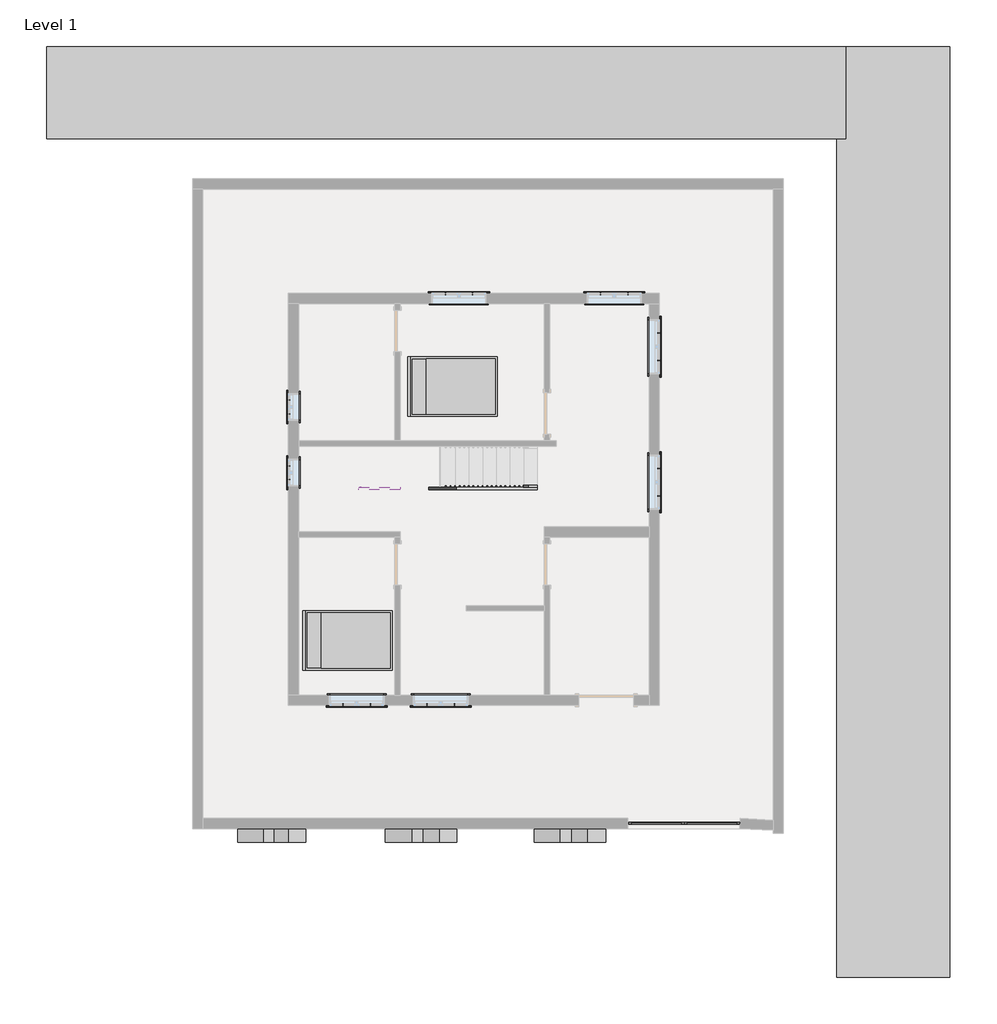
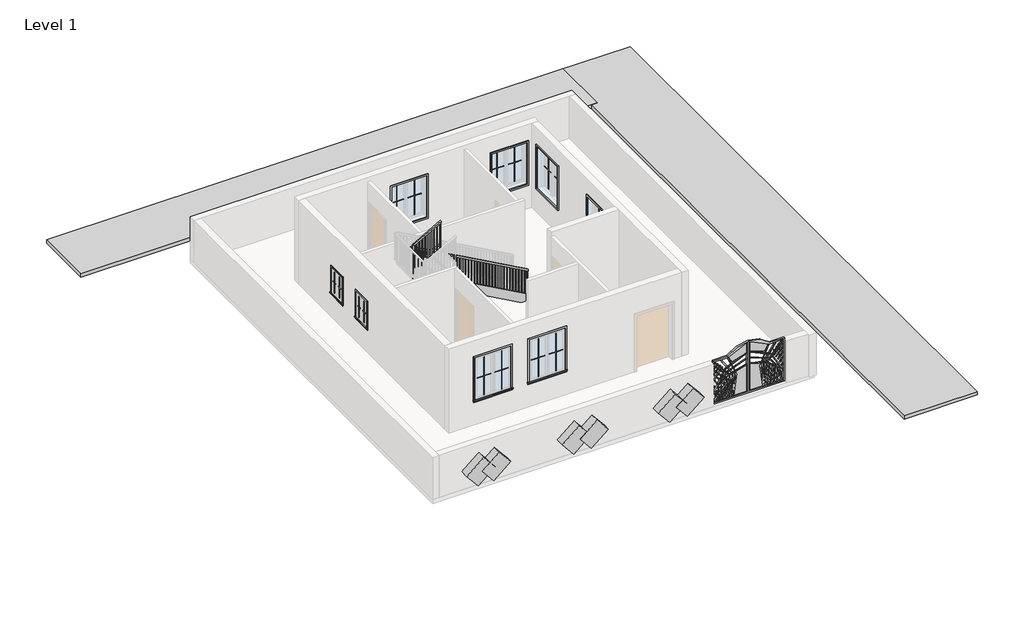
# One storey, part 2 of 2: 35 proxies, 3 members, 2 furniture elements, 1 railing.
"""IFC4 building model written with IfcOpenShell, lengths in millimetres."""

from ifc_helpers import new_model, si_unit, frame, origin, place, context, project, spatial, polyline, outline, extrude, faceted_brep, transform, mapped, element, save
from components import generic_models_6bc30956, generic_models_1_generic_models_1_8d9aa75c, generic_models_2_generic_models_2_aa56fe40, muntin_pattern_2x2_muntin_pattern_2x2_53152e2c, muntin_pattern_2x2_muntin_pattern_2x2_e8f3e573, muntin_pattern_2x2_muntin_pattern_2x2_6dad3731, muntin_pattern_2x2_muntin_pattern_2x2_a30a3345, trim_window_exterior_flat_with_sill_a665a915, trim_window_exterior_flat_with_sill_92b9b949, trim_window_interior_flat_picture_frame_d485c387, trim_window_interior_flat_picture_frame_3bb882cf, bed_17739_bed_17739_15c61121

model = new_model("IFC4")

# Units and contexts
model_context = context("Model", 3, world=origin())
ifc_project = project(units=[si_unit("LENGTHUNIT", "METRE", prefix="MILLI")], contexts=[model_context])

# Site, building, storey
site = spatial("IfcSite", under=ifc_project)
building = spatial("IfcBuilding", under=site)
storey = spatial("IfcBuildingStorey", under=building, Name="Level 1", Elevation=0.0)

# Proxies
placement = place(None, origin())
generic_models_shape = generic_models_6bc30956(model_context)
element("IfcBuildingElementProxy", 1, Name="Generic Models", at=placement, inside=storey, context=model_context, shape_type="MappedRepresentation", body=[
    mapped(generic_models_shape, transform((10047.0296029, 3046.038256, 0.0), x_axis=(1.0, 0.0, 0.0), y_axis=(0.0, 1.0, 0.0), z_axis=(0.0, 0.0, 1.0))),
])
generic_models_1_generic_models_1_shape = generic_models_1_generic_models_1_8d9aa75c(model_context)
element("IfcBuildingElementProxy", 2, Name="Generic Models 1 : Generic Models 1", ObjectType="Generic Models 1 : Generic Models 1", at=placement, inside=storey, context=model_context, shape_type="MappedRepresentation", body=[
    mapped(generic_models_1_generic_models_1_shape, transform((0.0, 0.0, 0.0), x_axis=(1.0, 0.0, 0.0), y_axis=(0.0, 1.0, 0.0), z_axis=(0.0, 0.0, 1.0))),
])
generic_models_2_generic_models_2_shape = generic_models_2_generic_models_2_aa56fe40(model_context)
element("IfcBuildingElementProxy", 3, Name="Generic Models 2 : Generic Models 2", ObjectType="Generic Models 2 : Generic Models 2", at=placement, inside=storey, context=model_context, shape_type="MappedRepresentation", body=[
    mapped(generic_models_2_generic_models_2_shape, transform((0.0, 0.0, 0.0), x_axis=(1.0, 0.0, 0.0), y_axis=(0.0, 1.0, 0.0), z_axis=(0.0, 0.0, 1.0))),
])
muntin_pattern_2x2_muntin_pattern_2x2_shape = muntin_pattern_2x2_muntin_pattern_2x2_53152e2c(model_context)
element("IfcBuildingElementProxy", 4, Name="Muntin Pattern_2x2 : Muntin Pattern_2x2", ObjectType="Muntin Pattern_2x2 : Muntin Pattern_2x2", at=placement, inside=storey, context=model_context, shape_type="MappedRepresentation", body=[
    mapped(muntin_pattern_2x2_muntin_pattern_2x2_shape, transform((1279.525, 12101.9997886, 984.25), x_axis=(0.0, 1.0, 0.0), y_axis=(-1.0, 0.0, 0.0), z_axis=(0.0, 0.0, 1.0))),
])
element("IfcBuildingElementProxy", 5, Name="Muntin Pattern_2x2 : Muntin Pattern_2x2", ObjectType="Muntin Pattern_2x2 : Muntin Pattern_2x2", at=placement, inside=storey, context=model_context, shape_type="MappedRepresentation", body=[
    mapped(muntin_pattern_2x2_muntin_pattern_2x2_shape, transform((1279.525, 10644.6747886, 984.25), x_axis=(0.0, 1.0, 0.0), y_axis=(-1.0, 0.0, 0.0), z_axis=(0.0, 0.0, 1.0))),
])
muntin_pattern_2x2_muntin_pattern_2x2_2_shape = muntin_pattern_2x2_muntin_pattern_2x2_e8f3e573(model_context)
element("IfcBuildingElementProxy", 6, Name="Muntin Pattern_2x2 : Muntin Pattern_2x2", ObjectType="Muntin Pattern_2x2 : Muntin Pattern_2x2", at=placement, inside=storey, context=model_context, shape_type="MappedRepresentation", body=[
    mapped(muntin_pattern_2x2_muntin_pattern_2x2_2_shape, transform((1279.525, 12403.6247886, 984.25), x_axis=(0.0, -1.0, 0.0), y_axis=(1.0, 0.0, 0.0), z_axis=(0.0, 0.0, 1.0))),
])
element("IfcBuildingElementProxy", 7, Name="Muntin Pattern_2x2 : Muntin Pattern_2x2", ObjectType="Muntin Pattern_2x2 : Muntin Pattern_2x2", at=placement, inside=storey, context=model_context, shape_type="MappedRepresentation", body=[
    mapped(muntin_pattern_2x2_muntin_pattern_2x2_2_shape, transform((1279.525, 10946.2997886, 984.25), x_axis=(0.0, -1.0, 0.0), y_axis=(1.0, 0.0, 0.0), z_axis=(0.0, 0.0, 1.0))),
])
muntin_pattern_2x2_muntin_pattern_2x2_3_shape = muntin_pattern_2x2_muntin_pattern_2x2_6dad3731(model_context)
element("IfcBuildingElementProxy", 8, Name="Muntin Pattern_2x2 : Muntin Pattern_2x2", ObjectType="Muntin Pattern_2x2 : Muntin Pattern_2x2", at=placement, inside=storey, context=model_context, shape_type="MappedRepresentation", body=[
    mapped(muntin_pattern_2x2_muntin_pattern_2x2_3_shape, transform((9490.075, 13892.6997886, 984.25), x_axis=(0.0, -1.0, 0.0), y_axis=(1.0, 0.0, 0.0), z_axis=(0.0, 0.0, 1.0))),
])
element("IfcBuildingElementProxy", 9, Name="Muntin Pattern_2x2 : Muntin Pattern_2x2", ObjectType="Muntin Pattern_2x2 : Muntin Pattern_2x2", at=placement, inside=storey, context=model_context, shape_type="MappedRepresentation", body=[
    mapped(muntin_pattern_2x2_muntin_pattern_2x2_3_shape, transform((8193.0875, 14767.4122886, 984.25), x_axis=(1.0, 0.0, 0.0), y_axis=(0.0, 1.0, 0.0), z_axis=(0.0, 0.0, 1.0))),
])
element("IfcBuildingElementProxy", 10, Name="Muntin Pattern_2x2 : Muntin Pattern_2x2", ObjectType="Muntin Pattern_2x2 : Muntin Pattern_2x2", at=placement, inside=storey, context=model_context, shape_type="MappedRepresentation", body=[
    mapped(muntin_pattern_2x2_muntin_pattern_2x2_3_shape, transform((4749.8, 14767.4122886, 984.25), x_axis=(1.0, 0.0, 0.0), y_axis=(0.0, 1.0, 0.0), z_axis=(0.0, 0.0, 1.0))),
])
element("IfcBuildingElementProxy", 11, Name="Muntin Pattern_2x2 : Muntin Pattern_2x2", ObjectType="Muntin Pattern_2x2 : Muntin Pattern_2x2", at=placement, inside=storey, context=model_context, shape_type="MappedRepresentation", body=[
    mapped(muntin_pattern_2x2_muntin_pattern_2x2_3_shape, transform((9490.075, 10889.1497886, 984.25), x_axis=(0.0, -1.0, 0.0), y_axis=(1.0, 0.0, 0.0), z_axis=(0.0, 0.0, 1.0))),
])
element("IfcBuildingElementProxy", 12, Name="Muntin Pattern_2x2 : Muntin Pattern_2x2", ObjectType="Muntin Pattern_2x2 : Muntin Pattern_2x2", at=placement, inside=storey, context=model_context, shape_type="MappedRepresentation", body=[
    mapped(muntin_pattern_2x2_muntin_pattern_2x2_3_shape, transform((4950.6207347, 5642.4622886, 984.25), x_axis=(-1.0, 0.0, 0.0), y_axis=(0.0, -1.0, 0.0), z_axis=(0.0, 0.0, 1.0))),
])
element("IfcBuildingElementProxy", 13, Name="Muntin Pattern_2x2 : Muntin Pattern_2x2", ObjectType="Muntin Pattern_2x2 : Muntin Pattern_2x2", at=placement, inside=storey, context=model_context, shape_type="MappedRepresentation", body=[
    mapped(muntin_pattern_2x2_muntin_pattern_2x2_3_shape, transform((3086.1019847, 5642.4622886, 984.25), x_axis=(-1.0, 0.0, 0.0), y_axis=(0.0, -1.0, 0.0), z_axis=(0.0, 0.0, 1.0))),
])
muntin_pattern_2x2_muntin_pattern_2x2_4_shape = muntin_pattern_2x2_muntin_pattern_2x2_a30a3345(model_context)
element("IfcBuildingElementProxy", 14, Name="Muntin Pattern_2x2 : Muntin Pattern_2x2", ObjectType="Muntin Pattern_2x2 : Muntin Pattern_2x2", at=placement, inside=storey, context=model_context, shape_type="MappedRepresentation", body=[
    mapped(muntin_pattern_2x2_muntin_pattern_2x2_4_shape, transform((9490.075, 13286.2747886, 984.25), x_axis=(0.0, 1.0, 0.0), y_axis=(-1.0, 0.0, 0.0), z_axis=(0.0, 0.0, 1.0))),
])
element("IfcBuildingElementProxy", 15, Name="Muntin Pattern_2x2 : Muntin Pattern_2x2", ObjectType="Muntin Pattern_2x2 : Muntin Pattern_2x2", at=placement, inside=storey, context=model_context, shape_type="MappedRepresentation", body=[
    mapped(muntin_pattern_2x2_muntin_pattern_2x2_4_shape, transform((8799.5125, 14767.4122886, 984.25), x_axis=(-1.0, 0.0, 0.0), y_axis=(0.0, -1.0, 0.0), z_axis=(0.0, 0.0, 1.0))),
])
element("IfcBuildingElementProxy", 16, Name="Muntin Pattern_2x2 : Muntin Pattern_2x2", ObjectType="Muntin Pattern_2x2 : Muntin Pattern_2x2", at=placement, inside=storey, context=model_context, shape_type="MappedRepresentation", body=[
    mapped(muntin_pattern_2x2_muntin_pattern_2x2_4_shape, transform((5356.225, 14767.4122886, 984.25), x_axis=(-1.0, 0.0, 0.0), y_axis=(0.0, -1.0, 0.0), z_axis=(0.0, 0.0, 1.0))),
])
element("IfcBuildingElementProxy", 17, Name="Muntin Pattern_2x2 : Muntin Pattern_2x2", ObjectType="Muntin Pattern_2x2 : Muntin Pattern_2x2", at=placement, inside=storey, context=model_context, shape_type="MappedRepresentation", body=[
    mapped(muntin_pattern_2x2_muntin_pattern_2x2_4_shape, transform((9490.075, 10282.7247886, 984.25), x_axis=(0.0, 1.0, 0.0), y_axis=(-1.0, 0.0, 0.0), z_axis=(0.0, 0.0, 1.0))),
])
element("IfcBuildingElementProxy", 18, Name="Muntin Pattern_2x2 : Muntin Pattern_2x2", ObjectType="Muntin Pattern_2x2 : Muntin Pattern_2x2", at=placement, inside=storey, context=model_context, shape_type="MappedRepresentation", body=[
    mapped(muntin_pattern_2x2_muntin_pattern_2x2_4_shape, transform((4344.1957347, 5642.4622886, 984.25), x_axis=(1.0, 0.0, 0.0), y_axis=(0.0, 1.0, 0.0), z_axis=(0.0, 0.0, 1.0))),
])
element("IfcBuildingElementProxy", 19, Name="Muntin Pattern_2x2 : Muntin Pattern_2x2", ObjectType="Muntin Pattern_2x2 : Muntin Pattern_2x2", at=placement, inside=storey, context=model_context, shape_type="MappedRepresentation", body=[
    mapped(muntin_pattern_2x2_muntin_pattern_2x2_4_shape, transform((2479.6769847, 5642.4622886, 984.25), x_axis=(1.0, 0.0, 0.0), y_axis=(0.0, 1.0, 0.0), z_axis=(0.0, 0.0, 1.0))),
])
trim_window_exterior_flat_with_sill_shape = trim_window_exterior_flat_with_sill_a665a915(model_context)
element("IfcBuildingElementProxy", 20, Name="Trim-Window-Exterior-Flat : with Sill", ObjectType="Trim-Window-Exterior-Flat : with Sill", at=placement, inside=storey, context=model_context, shape_type="MappedRepresentation", body=[
    mapped(trim_window_exterior_flat_with_sill_shape, transform((1270.0, 12252.8122886, 1828.8), x_axis=(0.0, -1.0, 0.0), y_axis=(0.0, 0.0, 1.0), z_axis=(-1.0, 0.0, 0.0))),
])
element("IfcBuildingElementProxy", 21, Name="Trim-Window-Exterior-Flat : with Sill", ObjectType="Trim-Window-Exterior-Flat : with Sill", at=placement, inside=storey, context=model_context, shape_type="MappedRepresentation", body=[
    mapped(trim_window_exterior_flat_with_sill_shape, transform((1270.0, 10795.4872886, 1828.8), x_axis=(0.0, -1.0, 0.0), y_axis=(0.0, 0.0, 1.0), z_axis=(-1.0, 0.0, 0.0))),
])
trim_window_exterior_flat_with_sill_2_shape = trim_window_exterior_flat_with_sill_92b9b949(model_context)
element("IfcBuildingElementProxy", 22, Name="Trim-Window-Exterior-Flat : with Sill", ObjectType="Trim-Window-Exterior-Flat : with Sill", at=placement, inside=storey, context=model_context, shape_type="MappedRepresentation", body=[
    mapped(trim_window_exterior_flat_with_sill_2_shape, transform((9499.6, 13589.4872886, 2438.4), x_axis=(0.0, 1.0, 0.0), y_axis=(0.0, 0.0, 1.0), z_axis=(1.0, 0.0, 0.0))),
])
element("IfcBuildingElementProxy", 23, Name="Trim-Window-Exterior-Flat : with Sill", ObjectType="Trim-Window-Exterior-Flat : with Sill", at=placement, inside=storey, context=model_context, shape_type="MappedRepresentation", body=[
    mapped(trim_window_exterior_flat_with_sill_2_shape, transform((8496.3, 14776.9372886, 2438.4), x_axis=(-1.0, 0.0, 0.0), y_axis=(0.0, 0.0, 1.0), z_axis=(0.0, 1.0, 0.0))),
])
element("IfcBuildingElementProxy", 24, Name="Trim-Window-Exterior-Flat : with Sill", ObjectType="Trim-Window-Exterior-Flat : with Sill", at=placement, inside=storey, context=model_context, shape_type="MappedRepresentation", body=[
    mapped(trim_window_exterior_flat_with_sill_2_shape, transform((5053.0125, 14776.9372886, 2438.4), x_axis=(-1.0, 0.0, 0.0), y_axis=(0.0, 0.0, 1.0), z_axis=(0.0, 1.0, 0.0))),
])
element("IfcBuildingElementProxy", 25, Name="Trim-Window-Exterior-Flat : with Sill", ObjectType="Trim-Window-Exterior-Flat : with Sill", at=placement, inside=storey, context=model_context, shape_type="MappedRepresentation", body=[
    mapped(trim_window_exterior_flat_with_sill_2_shape, transform((9499.6, 10585.9372886, 2438.4), x_axis=(0.0, 1.0, 0.0), y_axis=(0.0, 0.0, 1.0), z_axis=(1.0, 0.0, 0.0))),
])
element("IfcBuildingElementProxy", 26, Name="Trim-Window-Exterior-Flat : with Sill", ObjectType="Trim-Window-Exterior-Flat : with Sill", at=placement, inside=storey, context=model_context, shape_type="MappedRepresentation", body=[
    mapped(trim_window_exterior_flat_with_sill_2_shape, transform((4647.4082347, 5632.9372886, 2438.4), x_axis=(1.0, 0.0, 0.0), y_axis=(0.0, 0.0, 1.0), z_axis=(0.0, -1.0, 0.0))),
])
element("IfcBuildingElementProxy", 27, Name="Trim-Window-Exterior-Flat : with Sill", ObjectType="Trim-Window-Exterior-Flat : with Sill", at=placement, inside=storey, context=model_context, shape_type="MappedRepresentation", body=[
    mapped(trim_window_exterior_flat_with_sill_2_shape, transform((2782.8894847, 5632.9372886, 2438.4), x_axis=(1.0, 0.0, 0.0), y_axis=(0.0, 0.0, 1.0), z_axis=(0.0, -1.0, 0.0))),
])
trim_window_interior_flat_picture_frame_shape = trim_window_interior_flat_picture_frame_d485c387(model_context)
element("IfcBuildingElementProxy", 28, Name="Trim-Window-Interior-Flat : Picture Frame", ObjectType="Trim-Window-Interior-Flat : Picture Frame", at=placement, inside=storey, context=model_context, shape_type="MappedRepresentation", body=[
    mapped(trim_window_interior_flat_picture_frame_shape, transform((1498.6, 12252.8122886, 1828.8), x_axis=(0.0, 1.0, 0.0), y_axis=(0.0, 0.0, 1.0), z_axis=(1.0, 0.0, 0.0))),
])
element("IfcBuildingElementProxy", 29, Name="Trim-Window-Interior-Flat : Picture Frame", ObjectType="Trim-Window-Interior-Flat : Picture Frame", at=placement, inside=storey, context=model_context, shape_type="MappedRepresentation", body=[
    mapped(trim_window_interior_flat_picture_frame_shape, transform((1498.6, 10795.4872886, 1828.8), x_axis=(0.0, 1.0, 0.0), y_axis=(0.0, 0.0, 1.0), z_axis=(1.0, 0.0, 0.0))),
])
trim_window_interior_flat_picture_frame_2_shape = trim_window_interior_flat_picture_frame_3bb882cf(model_context)
element("IfcBuildingElementProxy", 30, Name="Trim-Window-Interior-Flat : Picture Frame", ObjectType="Trim-Window-Interior-Flat : Picture Frame", at=placement, inside=storey, context=model_context, shape_type="MappedRepresentation", body=[
    mapped(trim_window_interior_flat_picture_frame_2_shape, transform((9271.0, 13589.4872886, 2438.4), x_axis=(0.0, -1.0, 0.0), y_axis=(0.0, 0.0, 1.0), z_axis=(-1.0, 0.0, 0.0))),
])
element("IfcBuildingElementProxy", 31, Name="Trim-Window-Interior-Flat : Picture Frame", ObjectType="Trim-Window-Interior-Flat : Picture Frame", at=placement, inside=storey, context=model_context, shape_type="MappedRepresentation", body=[
    mapped(trim_window_interior_flat_picture_frame_2_shape, transform((8496.3, 14548.3372886, 2438.4), x_axis=(1.0, 0.0, 0.0), y_axis=(0.0, 0.0, 1.0), z_axis=(0.0, -1.0, 0.0))),
])
element("IfcBuildingElementProxy", 32, Name="Trim-Window-Interior-Flat : Picture Frame", ObjectType="Trim-Window-Interior-Flat : Picture Frame", at=placement, inside=storey, context=model_context, shape_type="MappedRepresentation", body=[
    mapped(trim_window_interior_flat_picture_frame_2_shape, transform((5053.0125, 14548.3372886, 2438.4), x_axis=(1.0, 0.0, 0.0), y_axis=(0.0, 0.0, 1.0), z_axis=(0.0, -1.0, 0.0))),
])
element("IfcBuildingElementProxy", 33, Name="Trim-Window-Interior-Flat : Picture Frame", ObjectType="Trim-Window-Interior-Flat : Picture Frame", at=placement, inside=storey, context=model_context, shape_type="MappedRepresentation", body=[
    mapped(trim_window_interior_flat_picture_frame_2_shape, transform((9271.0, 10585.9372886, 2438.4), x_axis=(0.0, -1.0, 0.0), y_axis=(0.0, 0.0, 1.0), z_axis=(-1.0, 0.0, 0.0))),
])
element("IfcBuildingElementProxy", 34, Name="Trim-Window-Interior-Flat : Picture Frame", ObjectType="Trim-Window-Interior-Flat : Picture Frame", at=placement, inside=storey, context=model_context, shape_type="MappedRepresentation", body=[
    mapped(trim_window_interior_flat_picture_frame_2_shape, transform((4647.4082347, 5861.5372886, 2438.4), x_axis=(-1.0, 0.0, 0.0), y_axis=(0.0, 0.0, 1.0), z_axis=(0.0, 1.0, 0.0))),
])
element("IfcBuildingElementProxy", 35, Name="Trim-Window-Interior-Flat : Picture Frame", ObjectType="Trim-Window-Interior-Flat : Picture Frame", at=placement, inside=storey, context=model_context, shape_type="MappedRepresentation", body=[
    mapped(trim_window_interior_flat_picture_frame_2_shape, transform((2782.8894847, 5861.5372886, 2438.4), x_axis=(-1.0, 0.0, 0.0), y_axis=(0.0, 0.0, 1.0), z_axis=(0.0, 1.0, 0.0))),
])

# Furniture
bed_17739_bed_17739_shape = bed_17739_bed_17739_15c61121(model_context)
element("IfcFurniture", 36, ObjectType="Bed_17739 : Bed_17739", at=placement, inside=storey, context=model_context, shape_type="MappedRepresentation", body=[
    mapped(bed_17739_bed_17739_shape, transform((4933.95, 12706.8372886, 0.0), x_axis=(0.0, 1.0, 0.0), y_axis=(-1.0, 0.0, 0.0), z_axis=(0.0, 0.0, 1.0))),
])
element("IfcFurniture", 37, ObjectType="Bed_17739 : Bed_17739", at=placement, inside=storey, context=model_context, shape_type="MappedRepresentation", body=[
    mapped(bed_17739_bed_17739_shape, transform((2603.5, 7074.3872886, 0.0), x_axis=(0.0, 1.0, 0.0), y_axis=(-1.0, 0.0, 0.0), z_axis=(0.0, 0.0, 1.0))),
])

# Members
element("IfcMember", 38, ObjectType="Stringer - 2\" Width", at=placement, inside=storey, context=model_context, shape_type="SweptSolid", body=[
    extrude(outline(polyline([(0.0, 6794.5), (207.5983948, 6794.5), (2380.7095059, 2882.9), (2032.0308318, 2882.9), (0.0, 6540.5554972), (0.0, 6794.5)])), frame((0.0, 10420.8372886, 0.0), z_axis=(0.0, 1.0, 0.0), x_axis=(0.0, 0.0, 1.0)), (0.0, 0.0, 1.0), 50.8),
])
element("IfcMember", 39, ObjectType="Stringer - 2\" Width", at=placement, inside=storey, context=model_context, shape_type="SweptSolid", body=[
    extrude(outline(polyline([(2832.1, 10471.6372886), (2882.9, 10471.6372886), (2882.9, 10469.0972886), (2832.1, 10469.0972886), (2832.1, 10471.6372886)])), frame((0.0, 0.0, 2142.0666667), z_axis=(0.0, 0.0, 1.0), x_axis=(1.0, 0.0, 0.0)), (0.0, 0.0, 1.0), 304.8),
])
element("IfcMember", 40, ObjectType="Stringer - 2\" Width", at=placement, inside=storey, context=model_context, shape_type="SweptSolid", body=[
    extrude(outline(polyline([(2578.2650614, 2832.1), (2229.5863873, 2832.1), (2737.5874899, 3746.5019847), (3086.266164, 3746.5019847), (2578.2650614, 2832.1)])), frame((0.0, 10418.2972886, 0.0), z_axis=(0.0, 1.0, 0.0), x_axis=(0.0, 0.0, 1.0)), (0.0, 0.0, 1.0), 50.8),
])

# Railing
element("IfcRailing", 41, ObjectType="Handrail - Rectangular", at=placement, inside=storey, context=model_context, shape_type="SolidModel", body=[
    faceted_brep([(6794.5, 10471.6372886, 1083.7333333), (6794.5, 10471.6372886, 1025.620221), (6794.5, 10522.4372886, 1025.620221), (6794.5, 10522.4372886, 1083.7333333), (2908.3, 10471.6372886, 3242.7333333), (2857.5, 10471.6372886, 3212.8424432), (2857.5, 10522.4372886, 3212.8424432), (2908.3, 10522.4372886, 3242.7333333), (2908.3, 10471.6372886, 3285.0666667), (2857.5, 10471.6372886, 3234.2666667), (2857.5, 10522.4372886, 3234.2666667), (2908.3, 10522.4372886, 3285.0666667), (2832.1, 10471.6372886, 3285.0666667), (2832.1, 10471.6372886, 3234.2666667), (2781.3, 10522.4372886, 3234.2666667), (2781.3, 10522.4372886, 3285.0666667), (2832.1, 10395.4372886, 3285.0666667), (2832.1, 10395.4372886, 3234.2666667), (2781.3, 10395.4372886, 3234.2666667), (2781.3, 10395.4372886, 3285.0666667), (2832.1, 10392.8972886, 3285.0666667), (2781.3, 10392.8972886, 3285.0666667), (2781.3, 10392.8972886, 3234.2666667), (2832.1, 10392.8972886, 3234.2666667)], [[[0, 1, 2, 3]], [[1, 0, 4, 5]], [[2, 1, 5, 6]], [[3, 2, 6, 7]], [[0, 3, 7, 4]], [[5, 4, 8, 9]], [[6, 5, 9, 10]], [[7, 6, 10, 11]], [[4, 7, 11, 8]], [[9, 8, 12, 13]], [[10, 9, 13, 14]], [[11, 10, 14, 15]], [[8, 11, 15, 12]], [[13, 12, 16, 17]], [[14, 13, 17, 18]], [[15, 14, 18, 19]], [[12, 15, 19, 16]], [[20, 21, 22, 23]], [[17, 16, 20, 23]], [[18, 17, 23, 22]], [[19, 18, 22, 21]], [[16, 19, 21, 20]]]),
    faceted_brep([(2832.1, 10418.2972886, 3285.0666667), (2832.1, 10367.4972886, 3234.2666667), (2781.3, 10367.4972886, 3234.2666667), (2781.3, 10418.2972886, 3285.0666667), (2832.1, 10418.2972886, 3396.2869174), (2781.3, 10418.2972886, 3426.177839), (2781.3, 10367.4972886, 3426.177839), (2832.1, 10367.4972886, 3396.2869174)], [[[0, 1, 2, 3]], [[4, 5, 6, 7]], [[1, 0, 4, 7]], [[2, 1, 7, 6]], [[3, 2, 6, 5]], [[0, 3, 5, 4]]]),
    faceted_brep([(2781.3, 10418.2972886, 3426.177839), (2832.1, 10418.2972886, 3396.2869174), (2832.1, 10367.4972886, 3396.2869174), (2781.3, 10367.4972886, 3426.177839), (3746.5019847, 10418.2972886, 3962.4), (3746.5019847, 10367.4972886, 3962.4), (3746.5019847, 10367.4972886, 3904.2869174), (3746.5019847, 10418.2972886, 3904.2869174)], [[[0, 1, 2, 3]], [[4, 5, 6, 7]], [[1, 0, 4, 7]], [[2, 1, 7, 6]], [[3, 2, 6, 5]], [[0, 3, 5, 4]]]),
    extrude(outline(polyline([(3884.8838142, 3711.575), (2878.6666667, 3711.575), (2878.6666667, 3730.625), (3895.4671246, 3730.625), (3884.8838142, 3711.575)])), frame((0.0, 10383.3722886, 0.0), z_axis=(0.0, 1.0, 0.0), x_axis=(0.0, 0.0, 1.0)), (0.0, 0.0, 1.0), 19.05),
    extrude(outline(polyline([(3828.4394923, 3609.975), (2878.6666667, 3609.975), (2878.6666667, 3629.025), (3839.0228026, 3629.025), (3828.4394923, 3609.975)])), frame((0.0, 10383.3722886, 0.0), z_axis=(0.0, 1.0, 0.0), x_axis=(0.0, 0.0, 1.0)), (0.0, 0.0, 1.0), 19.05),
    extrude(outline(polyline([(3771.9951703, 3508.375), (2878.6666667, 3508.375), (2878.6666667, 3527.425), (3782.5784807, 3527.425), (3771.9951703, 3508.375)])), frame((0.0, 10383.3722886, 0.0), z_axis=(0.0, 1.0, 0.0), x_axis=(0.0, 0.0, 1.0)), (0.0, 0.0, 1.0), 19.05),
    extrude(outline(polyline([(3715.5504809, 3406.775), (2709.3333333, 3406.775), (2709.3333333, 3425.825), (3726.1337912, 3425.825), (3715.5504809, 3406.775)])), frame((0.0, 10383.3722886, 0.0), z_axis=(0.0, 1.0, 0.0), x_axis=(0.0, 0.0, 1.0)), (0.0, 0.0, 1.0), 19.05),
    extrude(outline(polyline([(3659.1061589, 3305.175), (2709.3333333, 3305.175), (2709.3333333, 3324.225), (3669.6894693, 3324.225), (3659.1061589, 3305.175)])), frame((0.0, 10383.3722886, 0.0), z_axis=(0.0, 1.0, 0.0), x_axis=(0.0, 0.0, 1.0)), (0.0, 0.0, 1.0), 19.05),
    extrude(outline(polyline([(3602.661837, 3203.575), (2709.3333333, 3203.575), (2709.3333333, 3222.625), (3613.2451474, 3222.625), (3602.661837, 3203.575)])), frame((0.0, 10383.3722886, 0.0), z_axis=(0.0, 1.0, 0.0), x_axis=(0.0, 0.0, 1.0)), (0.0, 0.0, 1.0), 19.05),
    extrude(outline(polyline([(3546.2171475, 3101.975), (2540.0, 3101.975), (2540.0, 3121.025), (3556.8004579, 3121.025), (3546.2171475, 3101.975)])), frame((0.0, 10383.3722886, 0.0), z_axis=(0.0, 1.0, 0.0), x_axis=(0.0, 0.0, 1.0)), (0.0, 0.0, 1.0), 19.05),
    extrude(outline(polyline([(3489.7728256, 3000.375), (2540.0, 3000.375), (2540.0, 3019.425), (3500.356136, 3019.425), (3489.7728256, 3000.375)])), frame((0.0, 10383.3722886, 0.0), z_axis=(0.0, 1.0, 0.0), x_axis=(0.0, 0.0, 1.0)), (0.0, 0.0, 1.0), 19.05),
    extrude(outline(polyline([(3433.3285037, 2898.775), (2540.0, 2898.775), (2540.0, 2917.825), (3443.911814, 2917.825), (3433.3285037, 2898.775)])), frame((0.0, 10383.3722886, 0.0), z_axis=(0.0, 1.0, 0.0), x_axis=(0.0, 0.0, 1.0)), (0.0, 0.0, 1.0), 19.05),
    extrude(outline(polyline([(2816.225, 10404.9622886), (2816.225, 10385.9122886), (2797.175, 10385.9122886), (2797.175, 10404.9622886), (2816.225, 10404.9622886)])), frame((0.0, 0.0, 2370.6666667), z_axis=(0.0, 0.0, 1.0), x_axis=(1.0, 0.0, 0.0)), (0.0, 0.0, 1.0), 863.6),
    extrude(outline(polyline([(2841.625, 10487.5122886), (2822.575, 10487.5122886), (2822.575, 10506.5622886), (2841.625, 10506.5622886), (2841.625, 10487.5122886)])), frame((0.0, 0.0, 2370.6666667), z_axis=(0.0, 0.0, 1.0), x_axis=(1.0, 0.0, 0.0)), (0.0, 0.0, 1.0), 863.6),
    extrude(outline(polyline([(3175.8007765, 2924.175), (2201.3333333, 2924.175), (2201.3333333, 2943.225), (3165.2174432, 2943.225), (3175.8007765, 2924.175)])), frame((0.0, 10487.5122886, 0.0), z_axis=(0.0, 1.0, 0.0), x_axis=(0.0, 0.0, 1.0)), (0.0, 0.0, 1.0), 19.05),
    extrude(outline(polyline([(3119.3563321, 3025.775), (2201.3333333, 3025.775), (2201.3333333, 3044.825), (3108.7729988, 3044.825), (3119.3563321, 3025.775)])), frame((0.0, 10487.5122886, 0.0), z_axis=(0.0, 1.0, 0.0), x_axis=(0.0, 0.0, 1.0)), (0.0, 0.0, 1.0), 19.05),
    extrude(outline(polyline([(3062.9118876, 3127.375), (2201.3333333, 3127.375), (2201.3333333, 3146.425), (3052.3285543, 3146.425), (3062.9118876, 3127.375)])), frame((0.0, 10487.5122886, 0.0), z_axis=(0.0, 1.0, 0.0), x_axis=(0.0, 0.0, 1.0)), (0.0, 0.0, 1.0), 19.05),
    extrude(outline(polyline([(3006.4674432, 3228.975), (2032.0, 3228.975), (2032.0, 3248.025), (2995.8841099, 3248.025), (3006.4674432, 3228.975)])), frame((0.0, 10487.5122886, 0.0), z_axis=(0.0, 1.0, 0.0), x_axis=(0.0, 0.0, 1.0)), (0.0, 0.0, 1.0), 19.05),
    extrude(outline(polyline([(2950.0229988, 3330.575), (2032.0, 3330.575), (2032.0, 3349.625), (2939.4396654, 3349.625), (2950.0229988, 3330.575)])), frame((0.0, 10487.5122886, 0.0), z_axis=(0.0, 1.0, 0.0), x_axis=(0.0, 0.0, 1.0)), (0.0, 0.0, 1.0), 19.05),
    extrude(outline(polyline([(2893.5785543, 3432.175), (2032.0, 3432.175), (2032.0, 3451.225), (2882.995221, 3451.225), (2893.5785543, 3432.175)])), frame((0.0, 10487.5122886, 0.0), z_axis=(0.0, 1.0, 0.0), x_axis=(0.0, 0.0, 1.0)), (0.0, 0.0, 1.0), 19.05),
    extrude(outline(polyline([(2837.1341099, 3533.775), (1862.6666667, 3533.775), (1862.6666667, 3552.825), (2826.5507765, 3552.825), (2837.1341099, 3533.775)])), frame((0.0, 10487.5122886, 0.0), z_axis=(0.0, 1.0, 0.0), x_axis=(0.0, 0.0, 1.0)), (0.0, 0.0, 1.0), 19.05),
    extrude(outline(polyline([(2780.6896654, 3635.375), (1862.6666667, 3635.375), (1862.6666667, 3654.425), (2770.1063321, 3654.425), (2780.6896654, 3635.375)])), frame((0.0, 10487.5122886, 0.0), z_axis=(0.0, 1.0, 0.0), x_axis=(0.0, 0.0, 1.0)), (0.0, 0.0, 1.0), 19.05),
    extrude(outline(polyline([(2724.245221, 3736.975), (1862.6666667, 3736.975), (1862.6666667, 3756.025), (2713.6618876, 3756.025), (2724.245221, 3736.975)])), frame((0.0, 10487.5122886, 0.0), z_axis=(0.0, 1.0, 0.0), x_axis=(0.0, 0.0, 1.0)), (0.0, 0.0, 1.0), 19.05),
    extrude(outline(polyline([(2667.8007765, 3838.575), (1693.3333333, 3838.575), (1693.3333333, 3857.625), (2657.2174432, 3857.625), (2667.8007765, 3838.575)])), frame((0.0, 10487.5122886, 0.0), z_axis=(0.0, 1.0, 0.0), x_axis=(0.0, 0.0, 1.0)), (0.0, 0.0, 1.0), 19.05),
    extrude(outline(polyline([(2611.3563321, 3940.175), (1693.3333333, 3940.175), (1693.3333333, 3959.225), (2600.7729988, 3959.225), (2611.3563321, 3940.175)])), frame((0.0, 10487.5122886, 0.0), z_axis=(0.0, 1.0, 0.0), x_axis=(0.0, 0.0, 1.0)), (0.0, 0.0, 1.0), 19.05),
    extrude(outline(polyline([(2554.9118876, 4041.775), (1693.3333333, 4041.775), (1693.3333333, 4060.825), (2544.3285543, 4060.825), (2554.9118876, 4041.775)])), frame((0.0, 10487.5122886, 0.0), z_axis=(0.0, 1.0, 0.0), x_axis=(0.0, 0.0, 1.0)), (0.0, 0.0, 1.0), 19.05),
    extrude(outline(polyline([(2498.4674432, 4143.375), (1524.0, 4143.375), (1524.0, 4162.425), (2487.8841099, 4162.425), (2498.4674432, 4143.375)])), frame((0.0, 10487.5122886, 0.0), z_axis=(0.0, 1.0, 0.0), x_axis=(0.0, 0.0, 1.0)), (0.0, 0.0, 1.0), 19.05),
    extrude(outline(polyline([(2442.0229988, 4244.975), (1524.0, 4244.975), (1524.0, 4264.025), (2431.4396654, 4264.025), (2442.0229988, 4244.975)])), frame((0.0, 10487.5122886, 0.0), z_axis=(0.0, 1.0, 0.0), x_axis=(0.0, 0.0, 1.0)), (0.0, 0.0, 1.0), 19.05),
    extrude(outline(polyline([(2385.5785543, 4346.575), (1524.0, 4346.575), (1524.0, 4365.625), (2374.995221, 4365.625), (2385.5785543, 4346.575)])), frame((0.0, 10487.5122886, 0.0), z_axis=(0.0, 1.0, 0.0), x_axis=(0.0, 0.0, 1.0)), (0.0, 0.0, 1.0), 19.05),
    extrude(outline(polyline([(2329.1341099, 4448.175), (1354.6666667, 4448.175), (1354.6666667, 4467.225), (2318.5507765, 4467.225), (2329.1341099, 4448.175)])), frame((0.0, 10487.5122886, 0.0), z_axis=(0.0, 1.0, 0.0), x_axis=(0.0, 0.0, 1.0)), (0.0, 0.0, 1.0), 19.05),
    extrude(outline(polyline([(2272.6896654, 4549.775), (1354.6666667, 4549.775), (1354.6666667, 4568.825), (2262.1063321, 4568.825), (2272.6896654, 4549.775)])), frame((0.0, 10487.5122886, 0.0), z_axis=(0.0, 1.0, 0.0), x_axis=(0.0, 0.0, 1.0)), (0.0, 0.0, 1.0), 19.05),
    extrude(outline(polyline([(2216.245221, 4651.375), (1354.6666667, 4651.375), (1354.6666667, 4670.425), (2205.6618876, 4670.425), (2216.245221, 4651.375)])), frame((0.0, 10487.5122886, 0.0), z_axis=(0.0, 1.0, 0.0), x_axis=(0.0, 0.0, 1.0)), (0.0, 0.0, 1.0), 19.05),
    extrude(outline(polyline([(2159.8007765, 4752.975), (1185.3333333, 4752.975), (1185.3333333, 4772.025), (2149.2174432, 4772.025), (2159.8007765, 4752.975)])), frame((0.0, 10487.5122886, 0.0), z_axis=(0.0, 1.0, 0.0), x_axis=(0.0, 0.0, 1.0)), (0.0, 0.0, 1.0), 19.05),
    extrude(outline(polyline([(2103.3563321, 4854.575), (1185.3333333, 4854.575), (1185.3333333, 4873.625), (2092.7729988, 4873.625), (2103.3563321, 4854.575)])), frame((0.0, 10487.5122886, 0.0), z_axis=(0.0, 1.0, 0.0), x_axis=(0.0, 0.0, 1.0)), (0.0, 0.0, 1.0), 19.05),
    extrude(outline(polyline([(2046.9118876, 4956.175), (1185.3333333, 4956.175), (1185.3333333, 4975.225), (2036.3285543, 4975.225), (2046.9118876, 4956.175)])), frame((0.0, 10487.5122886, 0.0), z_axis=(0.0, 1.0, 0.0), x_axis=(0.0, 0.0, 1.0)), (0.0, 0.0, 1.0), 19.05),
    extrude(outline(polyline([(1990.4674432, 5057.775), (1016.0, 5057.775), (1016.0, 5076.825), (1979.8841099, 5076.825), (1990.4674432, 5057.775)])), frame((0.0, 10487.5122886, 0.0), z_axis=(0.0, 1.0, 0.0), x_axis=(0.0, 0.0, 1.0)), (0.0, 0.0, 1.0), 19.05),
    extrude(outline(polyline([(1934.0229988, 5159.375), (1016.0, 5159.375), (1016.0, 5178.425), (1923.4396654, 5178.425), (1934.0229988, 5159.375)])), frame((0.0, 10487.5122886, 0.0), z_axis=(0.0, 1.0, 0.0), x_axis=(0.0, 0.0, 1.0)), (0.0, 0.0, 1.0), 19.05),
    extrude(outline(polyline([(1877.5785543, 5260.975), (1016.0, 5260.975), (1016.0, 5280.025), (1866.995221, 5280.025), (1877.5785543, 5260.975)])), frame((0.0, 10487.5122886, 0.0), z_axis=(0.0, 1.0, 0.0), x_axis=(0.0, 0.0, 1.0)), (0.0, 0.0, 1.0), 19.05),
    extrude(outline(polyline([(1821.1341099, 5362.575), (846.6666667, 5362.575), (846.6666667, 5381.625), (1810.5507765, 5381.625), (1821.1341099, 5362.575)])), frame((0.0, 10487.5122886, 0.0), z_axis=(0.0, 1.0, 0.0), x_axis=(0.0, 0.0, 1.0)), (0.0, 0.0, 1.0), 19.05),
    extrude(outline(polyline([(1764.6896654, 5464.175), (846.6666667, 5464.175), (846.6666667, 5483.225), (1754.1063321, 5483.225), (1764.6896654, 5464.175)])), frame((0.0, 10487.5122886, 0.0), z_axis=(0.0, 1.0, 0.0), x_axis=(0.0, 0.0, 1.0)), (0.0, 0.0, 1.0), 19.05),
    extrude(outline(polyline([(1708.245221, 5565.775), (846.6666667, 5565.775), (846.6666667, 5584.825), (1697.6618876, 5584.825), (1708.245221, 5565.775)])), frame((0.0, 10487.5122886, 0.0), z_axis=(0.0, 1.0, 0.0), x_axis=(0.0, 0.0, 1.0)), (0.0, 0.0, 1.0), 19.05),
    extrude(outline(polyline([(1651.8007765, 5667.375), (677.3333333, 5667.375), (677.3333333, 5686.425), (1641.2174432, 5686.425), (1651.8007765, 5667.375)])), frame((0.0, 10487.5122886, 0.0), z_axis=(0.0, 1.0, 0.0), x_axis=(0.0, 0.0, 1.0)), (0.0, 0.0, 1.0), 19.05),
    extrude(outline(polyline([(1595.3563321, 5768.975), (677.3333333, 5768.975), (677.3333333, 5788.025), (1584.7729988, 5788.025), (1595.3563321, 5768.975)])), frame((0.0, 10487.5122886, 0.0), z_axis=(0.0, 1.0, 0.0), x_axis=(0.0, 0.0, 1.0)), (0.0, 0.0, 1.0), 19.05),
    extrude(outline(polyline([(1538.9118876, 5870.575), (677.3333333, 5870.575), (677.3333333, 5889.625), (1528.3285543, 5889.625), (1538.9118876, 5870.575)])), frame((0.0, 10487.5122886, 0.0), z_axis=(0.0, 1.0, 0.0), x_axis=(0.0, 0.0, 1.0)), (0.0, 0.0, 1.0), 19.05),
    extrude(outline(polyline([(1482.4674432, 5972.175), (508.0, 5972.175), (508.0, 5991.225), (1471.8841099, 5991.225), (1482.4674432, 5972.175)])), frame((0.0, 10487.5122886, 0.0), z_axis=(0.0, 1.0, 0.0), x_axis=(0.0, 0.0, 1.0)), (0.0, 0.0, 1.0), 19.05),
    extrude(outline(polyline([(1426.0229988, 6073.775), (508.0, 6073.775), (508.0, 6092.825), (1415.4396654, 6092.825), (1426.0229988, 6073.775)])), frame((0.0, 10487.5122886, 0.0), z_axis=(0.0, 1.0, 0.0), x_axis=(0.0, 0.0, 1.0)), (0.0, 0.0, 1.0), 19.05),
    extrude(outline(polyline([(1369.5785543, 6175.375), (508.0, 6175.375), (508.0, 6194.425), (1358.995221, 6194.425), (1369.5785543, 6175.375)])), frame((0.0, 10487.5122886, 0.0), z_axis=(0.0, 1.0, 0.0), x_axis=(0.0, 0.0, 1.0)), (0.0, 0.0, 1.0), 19.05),
    extrude(outline(polyline([(1313.1341099, 6276.975), (338.6666667, 6276.975), (338.6666667, 6296.025), (1302.5507765, 6296.025), (1313.1341099, 6276.975)])), frame((0.0, 10487.5122886, 0.0), z_axis=(0.0, 1.0, 0.0), x_axis=(0.0, 0.0, 1.0)), (0.0, 0.0, 1.0), 19.05),
    extrude(outline(polyline([(1256.6896654, 6378.575), (338.6666667, 6378.575), (338.6666667, 6397.625), (1246.1063321, 6397.625), (1256.6896654, 6378.575)])), frame((0.0, 10487.5122886, 0.0), z_axis=(0.0, 1.0, 0.0), x_axis=(0.0, 0.0, 1.0)), (0.0, 0.0, 1.0), 19.05),
    extrude(outline(polyline([(1200.245221, 6480.175), (338.6666667, 6480.175), (338.6666667, 6499.225), (1189.6618876, 6499.225), (1200.245221, 6480.175)])), frame((0.0, 10487.5122886, 0.0), z_axis=(0.0, 1.0, 0.0), x_axis=(0.0, 0.0, 1.0)), (0.0, 0.0, 1.0), 19.05),
    extrude(outline(polyline([(1143.8007765, 6581.775), (169.3333333, 6581.775), (169.3333333, 6600.825), (1133.2174432, 6600.825), (1143.8007765, 6581.775)])), frame((0.0, 10487.5122886, 0.0), z_axis=(0.0, 1.0, 0.0), x_axis=(0.0, 0.0, 1.0)), (0.0, 0.0, 1.0), 19.05),
    extrude(outline(polyline([(1087.3563321, 6683.375), (169.3333333, 6683.375), (169.3333333, 6702.425), (1076.7729988, 6702.425), (1087.3563321, 6683.375)])), frame((0.0, 10487.5122886, 0.0), z_axis=(0.0, 1.0, 0.0), x_axis=(0.0, 0.0, 1.0)), (0.0, 0.0, 1.0), 19.05),
    extrude(outline(polyline([(2816.225, 10402.4222886), (2816.225, 10383.3722886), (2797.175, 10383.3722886), (2797.175, 10402.4222886), (2816.225, 10402.4222886)])), frame((0.0, 0.0, 2370.6666667), z_axis=(0.0, 0.0, 1.0), x_axis=(1.0, 0.0, 0.0)), (0.0, 0.0, 1.0), 863.6),
    extrude(outline(polyline([(2816.225, 10487.5122886), (2797.175, 10487.5122886), (2797.175, 10506.5622886), (2816.225, 10506.5622886), (2816.225, 10487.5122886)])), frame((0.0, 0.0, 2370.6666667), z_axis=(0.0, 0.0, 1.0), x_axis=(1.0, 0.0, 0.0)), (0.0, 0.0, 1.0), 863.6),
    extrude(outline(polyline([(3893.703607, 3727.4519847), (2878.6666667, 3727.4519847), (2878.6666667, 3746.5019847), (3904.2869174, 3746.5019847), (3893.703607, 3727.4519847)])), frame((0.0, 10383.3722886, 0.0), z_axis=(0.0, 1.0, 0.0), x_axis=(0.0, 0.0, 1.0)), (0.0, 0.0, 1.0), 19.05),
    extrude(outline(polyline([(1036.2035543, 6775.45), (169.3333333, 6775.45), (169.3333333, 6794.5), (1025.620221, 6794.5), (1036.2035543, 6775.45)])), frame((0.0, 10487.5122886, 0.0), z_axis=(0.0, 1.0, 0.0), x_axis=(0.0, 0.0, 1.0)), (0.0, 0.0, 1.0), 19.05),
])

save(model, "model.ifc")

# Revit data of these elements
# Type
#   m.s. sheet = none
#   2" x2" pipe = none
#   1"x1"pipe = none
#   Default Elevation = 0
# Type "Muntin Pattern_2x2 : Muntin Pattern_2x2"
#   Width [instance default] = 4' - 0"
#   Thickness = 0' - 0 1/2"
#   Height [instance default] = 4' - 0"
#   Distance = 0' - 0 3/4"
#   Interior Material [instance default] = none
#   Exterior Material [instance default] = none
#   Default Elevation = 0
# Type "Trim-Window-Exterior-Flat : with Sill"
#   Trim Width = 0' - 2 1/4"
#   Trim Thickness_Picture Frame = 0' - 1 1/4"
#   Trim Thickness_with Sill = 0' - 0 3/4"
#   Sill Thickness = 0' - 1 1/4"
#   Opening Width [instance default] = 2' - 0"
#   Opening Height [instance default] = 3' - 0"
#   Default Elevation = 4' - 0"
#   Sill = yes
#   Picture Frame = no
#   Trim Material [instance default] = none
# Type "Trim-Window-Interior-Flat : Picture Frame"
#   Trim Thickness_Picture Frame = 0' - 1 1/4"
#   Trim Width = 0' - 2 1/4"
#   Trim Thickness_with Sill = 0' - 0 3/4"
#   Sill Thickness = 0' - 1 1/4"
#   Opening Width [instance default] = 2' - 0"
#   Opening Height [instance default] = 3' - 0"
#   Default Elevation = 4' - 0"
#   Sill = no
#   Picture Frame = yes
#   Trim Material [instance default] = none
# Type "Bed_17739 : Bed_17739"
#   Default Elevation = 0
# Type "Handrail - Rectangular"
#   Assembly Code = "C2010400"
#   built-in parameter 1008612 = 0.0416667 (stored number, unit not read)
#   built-in parameter 1008611 = 0.0416667 (stored number, unit not read)
#   built-in parameter 1008609 = 0.333333 (stored number, unit not read)
#   built-in parameter 1008604 = 0.166667 (stored number, unit not read)
#   built-in parameter 1008603 = 0.166667 (stored number, unit not read)
#   Railing Height = 3' - 0"
#   built-in parameter 1008630 = 2
#   built-in parameter 1008610 = 2
#   built-in parameter 1008618 = Baluster - Square : 3/4"
# Element 1 (IfcBuildingElementProxy)
#   Phase Created = New Construction
# Element 2 (IfcBuildingElementProxy, "Generic Models 1 : Generic Models 1")
#   Phase Created = New Construction
#   Materials on its faces: "Carpet (1)"
# Element 3 (IfcBuildingElementProxy, "Generic Models 2 : Generic Models 2")
#   Phase Created = New Construction
# Elements 4, 5, 6, 7 (IfcBuildingElementProxy, "Muntin Pattern_2x2 : Muntin Pattern_2x2")
#   Width = 0' - 6 5/8"
#   Height = 2' - 6 1/2"
#   Interior Material = Wood - Stained
#   Exterior Material = Clad - White
#   Phase Created = New Construction
#   Materials on its faces: "Clad - White", "Wood - Stained"
# Elements 8, 9, 10, 11, 12, 13, 14, 15, 16, 17, 18, 19 (IfcBuildingElementProxy, "Muntin Pattern_2x2 : Muntin Pattern_2x2")
#   Width = 1' - 6 5/8"
#   Height = 4' - 6 1/2"
#   Interior Material = Wood - Stained
#   Exterior Material = Clad - White
#   Phase Created = New Construction
#   Materials on its faces: "Clad - White", "Wood - Stained"
# Elements 20, 21 (IfcBuildingElementProxy, "Trim-Window-Exterior-Flat : with Sill")
#   Opening Width = 2' - 0"
#   Opening Height = 3' - 0"
#   Trim Material = Clad - White
#   Phase Created = New Construction
#   Materials on its faces: "Clad - White"
# Elements 22, 23, 24, 25, 26, 27 (IfcBuildingElementProxy, "Trim-Window-Exterior-Flat : with Sill")
#   Opening Width = 4' - 0"
#   Opening Height = 5' - 0"
#   Trim Material = Clad - White
#   Phase Created = New Construction
#   Materials on its faces: "Clad - White"
# Elements 28, 29 (IfcBuildingElementProxy, "Trim-Window-Interior-Flat : Picture Frame")
#   Opening Width = 2' - 0"
#   Opening Height = 3' - 0"
#   Trim Material = Wood - Stained
#   Phase Created = New Construction
#   Materials on its faces: "Wood - Stained"
# Elements 30, 31, 32, 33, 34, 35 (IfcBuildingElementProxy, "Trim-Window-Interior-Flat : Picture Frame")
#   Opening Width = 4' - 0"
#   Opening Height = 5' - 0"
#   Trim Material = Wood - Stained
#   Phase Created = New Construction
#   Materials on its faces: "Wood - Stained"
# Elements 36, 37 (IfcFurniture, "Bed_17739 : Bed_17739")
#   Phase Created = New Construction
#   Materials on its faces: "legs", "sheets", "bed frame", "Blanket"
# Elements 38, 39, 40 (IfcMember, "Stringer - 2\" Width")
#   Phase Created = New Construction
# Element 41 (IfcRailing, "Handrail - Rectangular")
#   Phase Created = New Construction
# Materials
#   "Carpet (1)": class "Carpet", colour RGB 124 80 67, transparency 0, Description = "Interior finish", Cost = 0
#   "Clad - White": class "Wood", colour RGB 242 242 238, transparency 0, Cost = 0
#   "Wood - Stained": class "Wood", colour RGB 224 178 126, transparency 0, Cost = 0
#   "legs": colour RGB 90 73 37, transparency 0, Cost = 0
#   "sheets": colour RGB 200 195 176, transparency 0, Cost = 0
#   "bed frame": colour RGB 90 73 37, transparency 0, Cost = 0
#   "Blanket": class "System", colour RGB 59 0 1, transparency 0, Cost = 0
